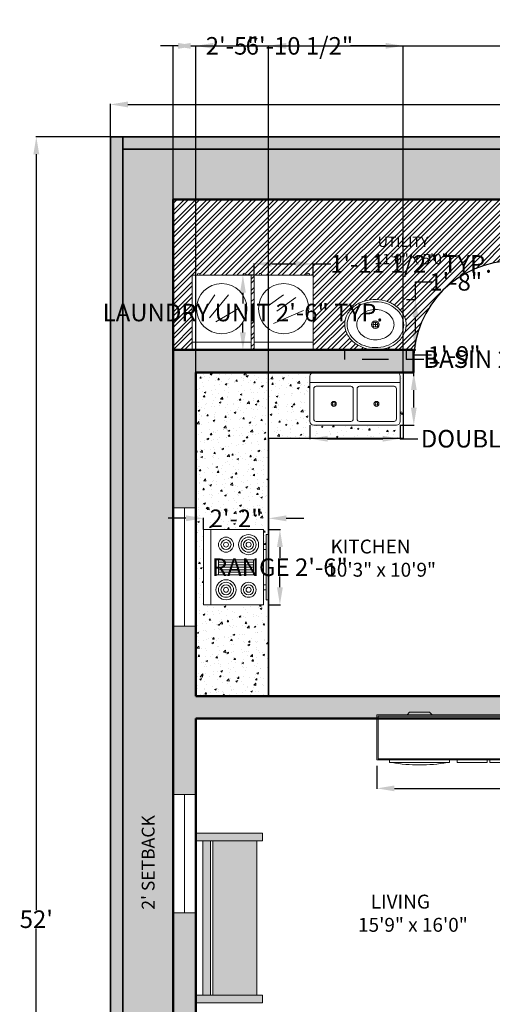
# Model space of a CAD drawing. Units: inches. Extents: x 319 to 870, y 210 to 995.
# Tile 4 of 6: x 336 to 524, y 603 to 995. Entities that reach past the tile are written whole.
import ezdxf

# ---------------------------------------------------------------- set-up
doc = ezdxf.new("R2010")
doc.units = ezdxf.units.IN
doc.header["$MEASUREMENT"] = 0
for name, color, linetype, lineweight in [('A-ANNO-DIMS', 2, 'Continuous', 18), ('A-ANNO-TEXT', 7, 'Continuous', 18), ('A-AREA-IDEN', 7, 'Continuous', 18), ('A-DOOR', 4, 'Continuous', 25), ('A-EQPM', 8, 'Continuous', 18), ('A-FLOR-CASE', 7, 'Continuous', 25), ('A-FLOR-CASE-PATT', 252, 'Continuous', 13), ('A-FLOR-FIXT', 9, 'Continuous', 18), ('A-FLOR-PATT', 252, 'Continuous', 13), ('A-FURN', 8, 'Continuous', 18), ('A-GLAZ', 4, 'Continuous', 18), ('A-WALL', 7, 'Continuous', 50), ('A-WALL-PATT', 8, 'Continuous', 13), ('C-PROP', 7, 'Continuous', 35), ('C-PROP-PATT', 8, 'Continuous', 13)]:
    doc.layers.add(name, color=color, linetype=linetype, lineweight=lineweight)
doc.layers.add('A-FURN-PATT', color=30, linetype='Continuous', lineweight=13, true_color=0xf7941d)
doc.layers.add('C-SITE-PATT', color=126, linetype='Continuous', lineweight=13, true_color=0x1e6f63)
doc.styles.get("Standard").update_dxf_attribs({"font": 'arial.ttf'})
doc.dimstyles.get("Standard").update_dxf_attribs({"dimtxt": 7, "dimasz": 7, "dimexe": 0.18, "dimexo": 0.0625, "dimgap": 0.09, "dimtad": 0, "dimtih": 1, "dimtoh": 1, "dimdec": 0, "dimzin": 0, "dimdsep": 46, "dimlunit": 3, "dimtxsty": 'Standard', "dimcen": 0.09, "dimadec": 0, "dimazin": 0, "dimtfac": 1, "dimtdec": 0, "dimtofl": 0, "dimtmove": 0, "dimatfit": 3, "dimfxl": 1, "dimtolj": 1, "dimtzin": 0, "dimarcsym": 0})

# ---------------------------------------------------------------- blocks, each defined once
blk = doc.blocks.new('Sink-double - 36 in top')
for p, q in [((-18, -4), (18, -4)), ((-0.75, -18.5), (-0.75, -6.5)), ((0.75, -6.5), (0.75, -18.5))]:
    blk.add_line(p, q)
for points in [[(-16.5, 0), (16.5, 0)], [(-18, -19.5), (-18, -1.5)], [(18, -1.5), (18, -19.5)], [(-16.5, -18.5), (-16.5, -6.5)], [(-15.5, -5.5), (-1.75, -5.5)], [(1.75, -5.5), (15.5, -5.5)], [(16.5, -6.5), (16.5, -18.5)], [(-1.75, -19.5), (-15.5, -19.5)], [(15.5, -19.5), (1.75, -19.5)], [(16.5, -21), (-16.5, -21)]]:
    blk.add_lwpolyline(points)
for centre, radius in [((-8.5, -12.5), 1), ((8.5, -12.5), 1), ((-8.5, -12.5), 0.5), ((8.5, -12.5), 0.5)]:
    blk.add_circle(centre, radius)
for centre, radius, start, end in [((-16.5, -1.5), 1.5, 90, 180), ((16.5, -1.5), 1.5, 0, 90), ((-15.5, -6.5), 1, 90, 180), ((-1.75, -6.5), 1, 0, 90), ((1.75, -6.5), 1, 90, 180), ((15.5, -6.5), 1, 0, 90), ((-16.5, -19.5), 1.5, 180, 270), ((-15.5, -18.5), 1, 180, 270), ((-1.75, -18.5), 1, 270, 0), ((1.75, -18.5), 1, 180, 270), ((15.5, -18.5), 1, 270, 0), ((16.5, -19.5), 1.5, 270, 0)]:
    blk.add_arc(centre, radius, start, end)
blk = doc.blocks.new('Range-Oven - 30 in top')
for p, q in [((0, -3), (30, -3)), ((12, -6), (18, -6)), ((13, -20), (13, -6)), ((14, -6), (14, -20)), ((15, -20), (15, -6)), ((16, -6), (16, -20)), ((17, -20), (17, -6)), ((18, -20), (12, -20)), ((6, -24), (6, -25)), ((8, -25), (8, -24)), ((22, -25), (22, -24)), ((24, -24), (24, -25))]:
    blk.add_line(p, q)
for points in [[(0, -24), (0, 0), (30, 0), (30, -24)], [(12, -21), (12, -5), (18, -5), (18, -21)], [(2, -26), (2, -25), (28, -25), (28, -26)]]:
    blk.add_lwpolyline(points, close=True)
for centre, radius in [((6, -9), 4), ((6, -9), 3), ((6, -9), 2), ((24, -9), 3), ((24, -9), 2), ((6, -9), 1), ((24, -9), 1), ((6, -18), 3), ((24, -18), 4), ((24, -18), 3), ((6, -18), 2), ((6, -18), 1), ((24, -18), 2), ((24, -18), 1)]:
    blk.add_circle(centre, radius)
blk = doc.blocks.new('Sink - Oval top')
for p, q in [((-1, 0), (1, 0)), ((0, 1), (0, -1))]:
    blk.add_line(p, q)
for points in [[(-12.23, 0.39, 0.117634), (-11.46, -3.36, 0.104469), (-8.88, -6.8, 0.090016), (-5.08, -9.07, 0.08192), (-0.32, -10.02, 0.08192), (4.49, -9.38, 0.090016), (8.42, -7.36, 0.104469), (11.22, -4.09, 0.117634), (12.23, -0.39, 0.117634), (11.46, 3.36, 0.104469), (8.88, 6.8, 0.090016), (5.08, 9.07, 0.08192), (0.32, 10.02, 0.08192), (-4.49, 9.38, 0.090016), (-8.42, 7.36, 0.104469), (-11.22, 4.09, 0.117634)], [(-11.29, 0.16, 0.118622), (-10.52, -3.25, 0.104678), (-8.07, -6.36, 0.089562), (-4.54, -8.37, 0.081185), (-0.13, -9.15, 0.081185), (4.3, -8.49, 0.089562), (7.89, -6.58, 0.104678), (10.42, -3.55, 0.118622), (11.29, -0.16, 0.118622), (10.52, 3.25, 0.104678), (8.07, 6.36, 0.089562), (4.54, 8.37, 0.081185), (0.13, 9.15, 0.081185), (-4.3, 8.49, 0.089562), (-7.89, 6.58, 0.104678), (-10.42, 3.55, 0.118622)], [(-7.42, 0.08, 0.118283), (-6.91, -2.17, 0.104607), (-5.29, -4.21, 0.089718), (-2.97, -5.53, 0.081436), (-0.07, -6.04, 0.081436), (2.84, -5.59, 0.089718), (5.2, -4.33, 0.104607), (6.86, -2.32, 0.118283), (7.42, -0.08, 0.118283), (6.91, 2.17, 0.104607), (5.29, 4.21, 0.089718), (2.97, 5.53, 0.081436), (0.07, 6.04, 0.081436), (-2.84, 5.59, 0.089718), (-5.2, 4.33, 0.104607), (-6.86, 2.32, 0.118283)]]:
    blk.add_lwpolyline(points, format="xyb", close=True)
for radius in [1.5, 1]:
    blk.add_circle((0, 0), radius)
blk = doc.blocks.new('*U12')
for p, q in [((0, 0), (0, -6)), ((-40, 0), (-40, -6))]:
    blk.add_line(p, q)
blk.add_lwpolyline([(0, 0), (0, 40), (-1.75, 40), (-1.75, 0)], close=True)
blk.add_arc((0, 0), 40, 90, 180)
blk = doc.blocks.new('Entertainment Center')
for p, q in [((-4, 0), (-5, -1)), ((4, 0), (-4, 0)), ((5, -1), (4, 0)), ((-17, -19), (-17, -1)), ((-17, -1), (43, -1)), ((-16.5, -18.5), (-16.5, -1.5)), ((-16.5, -1.5), (42.5, -1.5)), ((42.5, -1.5), (42.5, -18.5)), ((43, -1), (43, -19)), ((43, -19), (-17, -19)), ((42.5, -18.5), (-16.5, -18.5)), ((-12, -20), (-12, -19)), ((12, -19), (12, -20)), ((15, -20), (15, -19)), ((27, -19), (27, -20)), ((28, -20), (28, -19)), ((40, -19), (40, -20)), ((12, -20), (-12, -20)), ((27, -20), (15, -20)), ((40, -20), (28, -20))]:
    blk.add_line(p, q)
blk.add_arc((0, 40), 61, 259.6111, 280.3889)
blk = doc.blocks.new('*D22')
at = {"layer": 'A-ANNO-DIMS', "color": 0, "lineweight": -2, "transparency": 16777216}
for p, q in [((371.62, 948.67), (341.96, 948.67)), ((342.14, 941.67), (342.14, 640.33)), ((342.14, 331.67), (342.14, 633)), ((371.62, 324.67), (341.96, 324.67))]:
    blk.add_line(p, q, dxfattribs=at)
at = {"layer": 'A-ANNO-DIMS', "color": 0, "transparency": 16777216}
for points in [[(340.97, 941.67), (343.31, 941.67), (342.14, 948.67)], [(340.97, 331.67), (343.31, 331.67), (342.14, 324.67)]]:
    blk.add_solid(points, dxfattribs=at)
at = {"layer": 'Defpoints', "color": 0, "transparency": 16777216}
for p in [(371.68, 948.67), (342.14, 324.67), (371.68, 324.67)]:
    blk.add_point(p, dxfattribs=at)
at = {"layer": 'A-ANNO-DIMS', "color": 0, "transparency": 16777216, "insert": (342.14, 636.67), "char_height": 7, "attachment_point": 5}
blk.add_mtext("\\A1;52'", dxfattribs=at)
blk = doc.blocks.new('*D23')
at = {"layer": 'A-ANNO-DIMS', "color": 0, "lineweight": -2, "transparency": 16777216}
for p, q in [((371.68, 948.73), (371.68, 961.74)), ((378.68, 961.56), (575.66, 961.56)), ((784.68, 961.56), (587.71, 961.56)), ((791.68, 948.73), (791.68, 961.74))]:
    blk.add_line(p, q, dxfattribs=at)
at = {"layer": 'A-ANNO-DIMS', "color": 0, "transparency": 16777216}
for points in [[(378.68, 962.73), (378.68, 960.39), (371.68, 961.56)], [(784.68, 962.73), (784.68, 960.39), (791.68, 961.56)]]:
    blk.add_solid(points, dxfattribs=at)
at = {"layer": 'Defpoints', "color": 0, "transparency": 16777216}
for p in [(791.68, 961.56), (371.68, 948.67), (791.68, 948.67)]:
    blk.add_point(p, dxfattribs=at)
at = {"layer": 'A-ANNO-DIMS', "color": 0, "transparency": 16777216, "insert": (581.68, 961.56), "char_height": 7, "attachment_point": 5}
blk.add_mtext("\\A1;35'", dxfattribs=at)
blk = doc.blocks.new('EQPM-LAUNDRY-CABINET-DRUM')
for p, q in [((0, 0), (0, 29.82)), ((0, 29.82), (23.57, 29.82)), ((23.57, 29.82), (23.57, 0)), ((23.57, 3.06), (0, 3.06))]:
    blk.add_line(p, q)
blk.add_circle((11.78, 16.44), 10.02)
blk = doc.blocks.new('*D29')
at = {"layer": 'A-ANNO-DIMS', "color": 0, "lineweight": -2, "transparency": 16777216}
for p, q in [((477.94, 697.77), (477.94, 688.66)), ((537.94, 697.77), (537.94, 688.66)), ((484.94, 688.84), (530.94, 688.84)), ((537.94, 688.84), (544.94, 688.84))]:
    blk.add_line(p, q, dxfattribs=at)
at = {"layer": 'A-ANNO-DIMS', "color": 0, "transparency": 16777216}
for points in [[(484.94, 690), (484.94, 687.67), (477.94, 688.84)], [(530.94, 690), (530.94, 687.67), (537.94, 688.84)]]:
    blk.add_solid(points, dxfattribs=at)
at = {"layer": 'Defpoints', "color": 0, "transparency": 16777216}
for p in [(477.94, 697.84), (537.94, 697.84), (537.94, 688.84)]:
    blk.add_point(p, dxfattribs=at)
at = {"layer": 'A-ANNO-DIMS', "color": 0, "transparency": 16777216, "insert": (595.82, 688.84), "char_height": 7, "attachment_point": 5}
blk.add_mtext('\\A1;MEDIA UNIT 5\'-0" TYP.', dxfattribs=at)
blk = doc.blocks.new('*D41')
at = {"layer": 'A-ANNO-DIMS', "color": 0, "lineweight": -2, "transparency": 16777216}
for p, q in [((428.91, 893.49), (424.32, 893.49)), ((424.5, 886.49), (424.5, 882.24)), ((424.5, 870.67), (424.5, 874.92)), ((428.91, 863.67), (424.32, 863.67))]:
    blk.add_line(p, q, dxfattribs=at)
at = {"layer": 'A-ANNO-DIMS', "color": 0, "transparency": 16777216}
for points in [[(423.34, 886.49), (425.67, 886.49), (424.5, 893.49)], [(423.34, 870.67), (425.67, 870.67), (424.5, 863.67)]]:
    blk.add_solid(points, dxfattribs=at)
at = {"layer": 'Defpoints', "color": 0, "transparency": 16777216}
for p in [(424.5, 893.49), (428.98, 893.49), (428.98, 863.67)]:
    blk.add_point(p, dxfattribs=at)
at = {"layer": 'A-ANNO-DIMS', "color": 0, "transparency": 16777216, "insert": (424.5, 878.58), "char_height": 7, "attachment_point": 5}
blk.add_mtext('\\A1;LAUNDRY UNIT 2\'-6" TYP.', dxfattribs=at)
blk = doc.blocks.new('*D42')
at = {"layer": 'A-ANNO-DIMS', "color": 0, "lineweight": -2, "transparency": 16777216}
for p, q in [((428.98, 893.55), (428.98, 898.15)), ((435.98, 897.97), (445.54, 897.97)), ((452.54, 893.55), (452.54, 898.15)), ((452.54, 897.97), (459.54, 897.97))]:
    blk.add_line(p, q, dxfattribs=at)
at = {"layer": 'A-ANNO-DIMS', "color": 0, "transparency": 16777216}
for points in [[(435.98, 899.13), (435.98, 896.8), (428.98, 897.97)], [(445.54, 899.13), (445.54, 896.8), (452.54, 897.97)]]:
    blk.add_solid(points, dxfattribs=at)
at = {"layer": 'Defpoints', "color": 0, "transparency": 16777216}
for p in [(452.54, 897.97), (428.98, 893.49), (452.54, 893.49)]:
    blk.add_point(p, dxfattribs=at)
at = {"layer": 'A-ANNO-DIMS', "color": 0, "transparency": 16777216, "insert": (491.51, 897.97), "char_height": 7, "attachment_point": 5}
blk.add_mtext('\\A1;1\'-11 1/2" TYP.', dxfattribs=at)
blk = doc.blocks.new('*D43')
at = {"layer": 'A-ANNO-DIMS', "color": 0, "lineweight": -2, "transparency": 16777216}
for p, q in [((451.25, 833.61), (451.25, 828.09)), ((487.25, 833.61), (487.25, 828.09)), ((458.25, 828.27), (480.25, 828.27)), ((487.25, 828.27), (494.25, 828.27))]:
    blk.add_line(p, q, dxfattribs=at)
at = {"layer": 'A-ANNO-DIMS', "color": 0, "transparency": 16777216}
for points in [[(458.25, 829.44), (458.25, 827.1), (451.25, 828.27)], [(480.25, 829.44), (480.25, 827.1), (487.25, 828.27)]]:
    blk.add_solid(points, dxfattribs=at)
at = {"layer": 'Defpoints', "color": 0, "transparency": 16777216}
for p in [(451.25, 833.67), (487.25, 833.67), (487.25, 828.27)]:
    blk.add_point(p, dxfattribs=at)
at = {"layer": 'A-ANNO-DIMS', "color": 0, "transparency": 16777216, "insert": (537.71, 828.27), "char_height": 7, "attachment_point": 5}
blk.add_mtext('\\A1;DOUBLE SINK 3\'-0"', dxfattribs=at)
blk = doc.blocks.new('*D44')
at = {"layer": 'A-ANNO-DIMS', "color": 0, "lineweight": -2, "transparency": 16777216}
for p, q in [((492.65, 854.67), (492.65, 861.67)), ((492.65, 861.67), (499.65, 861.67)), ((487.31, 854.67), (492.83, 854.67)), ((492.65, 840.67), (492.65, 847.67)), ((487.31, 833.67), (492.83, 833.67))]:
    blk.add_line(p, q, dxfattribs=at)
at = {"layer": 'A-ANNO-DIMS', "color": 0, "transparency": 16777216}
for points in [[(491.49, 847.67), (493.82, 847.67), (492.65, 854.67)], [(491.49, 840.67), (493.82, 840.67), (492.65, 833.67)]]:
    blk.add_solid(points, dxfattribs=at)
at = {"layer": 'Defpoints', "color": 0, "transparency": 16777216}
for p in [(487.25, 854.67), (492.65, 854.67), (487.25, 833.67)]:
    blk.add_point(p, dxfattribs=at)
at = {"layer": 'A-ANNO-DIMS', "color": 0, "transparency": 16777216, "insert": (508.72, 861.67), "char_height": 7, "attachment_point": 5}
blk.add_mtext('\\A1;1\'-9"', dxfattribs=at)
blk = doc.blocks.new('*D45')
at = {"layer": 'A-ANNO-DIMS', "color": 0, "lineweight": -2, "transparency": 16777216}
for p, q in [((434.83, 792.03), (439.45, 792.03)), ((439.27, 785.03), (439.27, 780.74)), ((439.27, 769.03), (439.27, 773.32)), ((434.83, 762.03), (439.45, 762.03))]:
    blk.add_line(p, q, dxfattribs=at)
at = {"layer": 'A-ANNO-DIMS', "color": 0, "transparency": 16777216}
for points in [[(438.1, 785.03), (440.44, 785.03), (439.27, 792.03)], [(438.1, 769.03), (440.44, 769.03), (439.27, 762.03)]]:
    blk.add_solid(points, dxfattribs=at)
at = {"layer": 'Defpoints', "color": 0, "transparency": 16777216}
for p in [(434.77, 792.03), (439.27, 792.03), (434.77, 762.03)]:
    blk.add_point(p, dxfattribs=at)
at = {"layer": 'A-ANNO-DIMS', "color": 0, "transparency": 16777216, "insert": (439.27, 777.03), "char_height": 7, "attachment_point": 5}
blk.add_mtext('\\A1;RANGE 2\'-6"', dxfattribs=at)
blk = doc.blocks.new('*D46')
at = {"layer": 'A-ANNO-DIMS', "color": 0, "lineweight": -2, "transparency": 16777216}
for p, q in [((401.77, 796.53), (394.77, 796.53)), ((408.77, 792.09), (408.77, 796.71)), ((434.77, 792.09), (434.77, 796.71)), ((441.77, 796.53), (448.77, 796.53))]:
    blk.add_line(p, q, dxfattribs=at)
at = {"layer": 'A-ANNO-DIMS', "color": 0, "transparency": 16777216}
for points in [[(401.77, 797.7), (401.77, 795.36), (408.77, 796.53)], [(441.77, 797.7), (441.77, 795.36), (434.77, 796.53)]]:
    blk.add_solid(points, dxfattribs=at)
at = {"layer": 'Defpoints', "color": 0, "transparency": 16777216}
for p in [(408.77, 796.53), (408.77, 792.03), (434.77, 792.03)]:
    blk.add_point(p, dxfattribs=at)
at = {"layer": 'A-ANNO-DIMS', "color": 0, "transparency": 16777216, "insert": (421.77, 796.53), "char_height": 7, "attachment_point": 5}
blk.add_mtext('\\A1;2\'-2"', dxfattribs=at)
blk = doc.blocks.new('*D47')
at = {"layer": 'A-ANNO-DIMS', "color": 0, "lineweight": -2, "transparency": 16777216}
for p, q in [((465.06, 863.63), (465.06, 859.83)), ((472.06, 860.01), (482.61, 860.01)), ((489.61, 863.63), (489.61, 859.83)), ((489.61, 860.01), (496.61, 860.01))]:
    blk.add_line(p, q, dxfattribs=at)
at = {"layer": 'A-ANNO-DIMS', "color": 0, "transparency": 16777216}
for points in [[(472.06, 861.17), (472.06, 858.84), (465.06, 860.01)], [(482.61, 861.17), (482.61, 858.84), (489.61, 860.01)]]:
    blk.add_solid(points, dxfattribs=at)
at = {"layer": 'Defpoints', "color": 0, "transparency": 16777216}
for p in [(465.06, 863.69), (489.61, 863.69), (489.61, 860.01)]:
    blk.add_point(p, dxfattribs=at)
at = {"layer": 'A-ANNO-DIMS', "color": 0, "transparency": 16777216, "insert": (530.04, 860.01), "char_height": 7, "attachment_point": 5}
blk.add_mtext('\\A1;BASIN 2\'-0 1/2"', dxfattribs=at)
blk = doc.blocks.new('*D48')
at = {"layer": 'A-ANNO-DIMS', "color": 0, "lineweight": -2, "transparency": 16777216}
for p, q in [((493.3, 883.83), (493.3, 890.83)), ((493.3, 890.83), (500.3, 890.83)), ((489.68, 883.83), (493.48, 883.83)), ((493.3, 870.69), (493.3, 876.83)), ((489.68, 863.69), (493.48, 863.69))]:
    blk.add_line(p, q, dxfattribs=at)
at = {"layer": 'A-ANNO-DIMS', "color": 0, "transparency": 16777216}
for points in [[(492.13, 876.83), (494.46, 876.83), (493.3, 883.83)], [(492.13, 870.69), (494.46, 870.69), (493.3, 863.69)]]:
    blk.add_solid(points, dxfattribs=at)
at = {"layer": 'Defpoints', "color": 0, "transparency": 16777216}
for p in [(489.61, 883.83), (493.3, 883.83), (489.61, 863.69)]:
    blk.add_point(p, dxfattribs=at)
at = {"layer": 'A-ANNO-DIMS', "color": 0, "transparency": 16777216, "insert": (509.36, 890.83), "char_height": 7, "attachment_point": 5}
blk.add_mtext('\\A1;1\'-8"', dxfattribs=at)
blk = doc.blocks.new('*D49')
at = {"layer": 'A-ANNO-DIMS', "color": 0, "lineweight": -2, "transparency": 16777216}
for p, q in [((396.68, 923.73), (396.68, 985.1)), ((403.68, 984.92), (566.85, 984.92)), ((759.68, 984.92), (596.52, 984.92)), ((766.68, 923.73), (766.68, 985.1))]:
    blk.add_line(p, q, dxfattribs=at)
at = {"layer": 'A-ANNO-DIMS', "color": 0, "transparency": 16777216}
for points in [[(403.68, 986.09), (403.68, 983.75), (396.68, 984.92)], [(759.68, 986.09), (759.68, 983.75), (766.68, 984.92)]]:
    blk.add_solid(points, dxfattribs=at)
at = {"layer": 'Defpoints', "color": 0, "transparency": 16777216}
for p in [(766.68, 984.92), (396.68, 923.67), (766.68, 923.67)]:
    blk.add_point(p, dxfattribs=at)
at = {"layer": 'A-ANNO-DIMS', "color": 0, "transparency": 16777216, "insert": (581.68, 984.92), "char_height": 7, "attachment_point": 5}
blk.add_mtext('\\A1;30\'-10"', dxfattribs=at)
blk = doc.blocks.new('*D57')
at = {"layer": 'A-ANNO-DIMS', "color": 0, "lineweight": -2, "transparency": 16777216}
for p, q in [((405.68, 854.73), (405.68, 985.1)), ((412.68, 984.92), (426.76, 984.92)), ((481.42, 984.92), (467.34, 984.92)), ((488.42, 854.73), (488.42, 985.1))]:
    blk.add_line(p, q, dxfattribs=at)
at = {"layer": 'A-ANNO-DIMS', "color": 0, "transparency": 16777216}
for points in [[(412.68, 986.09), (412.68, 983.75), (405.68, 984.92)], [(481.42, 986.09), (481.42, 983.75), (488.42, 984.92)]]:
    blk.add_solid(points, dxfattribs=at)
at = {"layer": 'Defpoints', "color": 0, "transparency": 16777216}
for p in [(488.42, 984.92), (405.68, 854.67), (488.42, 854.67)]:
    blk.add_point(p, dxfattribs=at)
at = {"layer": 'A-ANNO-DIMS', "color": 0, "transparency": 16777216, "insert": (447.05, 984.92), "char_height": 7, "attachment_point": 5}
blk.add_mtext('\\A1;6\'-10 1/2"', dxfattribs=at)
blk = doc.blocks.new('*D58')
at = {"layer": 'A-ANNO-DIMS', "color": 0, "lineweight": -2, "transparency": 16777216}
for p, q in [((398.68, 984.92), (391.68, 984.92)), ((405.68, 725.73), (405.68, 985.1)), ((434.77, 725.73), (434.77, 985.1)), ((441.77, 984.92), (448.77, 984.92))]:
    blk.add_line(p, q, dxfattribs=at)
at = {"layer": 'A-ANNO-DIMS', "color": 0, "transparency": 16777216}
for points in [[(398.68, 986.09), (398.68, 983.75), (405.68, 984.92)], [(441.77, 986.09), (441.77, 983.75), (434.77, 984.92)]]:
    blk.add_solid(points, dxfattribs=at)
at = {"layer": 'Defpoints', "color": 0, "transparency": 16777216}
for p in [(434.77, 984.92), (405.68, 725.67), (434.77, 725.67)]:
    blk.add_point(p, dxfattribs=at)
at = {"layer": 'A-ANNO-DIMS', "color": 0, "transparency": 16777216, "insert": (420.23, 984.92), "char_height": 7, "attachment_point": 5}
blk.add_mtext('\\A1;2\'-5"', dxfattribs=at)

msp = doc.modelspace()

# ---------------------------------------------------------------- hatches: boundary and pattern name
at = {"layer": 'A-FLOR-CASE-PATT'}
h = msp.add_hatch(dxfattribs=at)
h.set_pattern_fill('AR-CONC', color=256)
h.set_pattern_definition([(50, (0, 0), (7.172602, -0.62752), [0.75, -8.25]), (355, (0, 0), (-1.387513, 7.52192), [0.6, -6.6]), (100.45144, (0.598, -0.052), (5.78509, 6.8944), [0.6374, -7.01142]), (46.1842, (0, 2), (10.67241, -1.65519), [1.125, -12.375]), (96.6356, (0.889, 1.862), (9.34662, 9.74119), [0.9561, -10.51714]), (351.1842, (0, 2), (9.34662, 9.74119), [0.9, -9.9]), (21, (1, 1.5), (5.96907, -4.02619), [0.75, -8.25]), (326, (1, 1.5), (2.433153, 7.2515), [0.6, -6.6]), (71.45144, (1.4974, 1.1645), (8.402224, 3.22531), [0.6374, -7.01142]), (37.5, (0, 0), (0.1215986, 3.3289385), [0, -6.52, 0, -6.7, 0, -6.625]), (7.5, (0, 0), (2.630695, 3.944117), [0, -3.82, 0, -6.37, 0, -2.525]), (327.5, (-2.23, 0), (5.338224, -0.225549), [0, -2.5, 0, -7.8, 0, -10.35]), (317.5, (-3.23, 0), (5.831862, 1.00105), [0, -3.25, 0, -5.18, 0, -7.35])])
h.paths.add_polyline_path([(405.68, 725.67), (434.77, 725.67), (434.77, 764.03), (433.77, 764.03), (433.77, 768.03), (432.77, 768.03), (432.77, 762.03), (408.77, 762.03), (408.77, 792.03), (432.77, 792.03), (432.77, 786.03), (433.77, 786.03), (433.77, 790.03), (434.77, 790.03), (434.77, 828.39), (488.42, 828.39), (488.42, 854.67), (485.75, 854.67, -0.414214), (487.25, 853.17), (487.25, 835.17, -0.414214), (485.75, 833.67), (452.75, 833.67, -0.414214), (451.25, 835.17), (451.25, 853.17, -0.414214), (452.75, 854.67), (405.68, 854.67)])
at = {"layer": 'A-FLOR-PATT'}
h = msp.add_hatch(dxfattribs=at)
h.set_pattern_fill('STEEL', color=256)
h.set_pattern_definition([(45, (0, 0), (-2.245064, 2.245064), []), (45, (0, 1.5875), (-2.245064, 2.245064), [])])
h.paths.add_polyline_path([(472.85, 883.14, -0.08192), (477.66, 883.77, -0.08192), (482.42, 882.83, -0.090016), (486.22, 880.56, -0.104469), (488.8, 877.12, -0.117634), (489.57, 873.36, -0.117634), (488.56, 869.67, -0.104469), (485.76, 866.4, -0.090016), (481.83, 864.38, -0.073818), (477.49, 863.73), (492.56, 863.67), (492.82, 863.67, -0.354003), (528.68, 898.98), (528.68, 923.67), (396.68, 923.67), (396.68, 863.67), (404.28, 863.67), (404.28, 893.49), (406.44, 893.49, -1.658066), (407.33, 893.49), (424.73, 893.49, -1.757253), (425.6, 893.49), (427.85, 893.49), (427.85, 863.67), (428.98, 863.67), (428.98, 893.49), (431.02, 893.49, -1.575486), (431.93, 893.49), (450.07, 893.49, -1.717768), (450.95, 893.49), (452.54, 893.49), (452.54, 863.67), (477.49, 863.73, -0.008053), (477.01, 863.74, -0.08192), (472.25, 864.69, -0.090016), (468.46, 866.95, -0.104469), (465.87, 870.4, -0.117634), (465.1, 874.15, -0.117634), (466.11, 877.85, -0.104469), (468.92, 881.12, -0.090016)])
h.paths.add_polyline_path([(475.31, 895.58), (505.85, 895.58), (505.85, 911.01), (475.31, 911.01)], flags=24)
at = {"layer": 'A-FURN-PATT'}
h = msp.add_hatch(color=256, dxfattribs=at)
h.dxf.hatch_style = 1
h.paths.add_polyline_path([(432.33, 667.94), (432.33, 670.94), (405.68, 670.94), (405.68, 667.94)])
h = msp.add_hatch(color=256, dxfattribs=at)
h.dxf.hatch_style = 1
h.paths.add_polyline_path([(411.58, 667.94), (408.53, 667.94), (408.53, 606.35), (411.58, 606.35)])
h = msp.add_hatch(color=256, dxfattribs=at)
h.dxf.hatch_style = 1
h.paths.add_polyline_path([(412.58, 606.35), (430.1, 606.35), (430.1, 667.94), (412.58, 667.94)])
h = msp.add_hatch(color=256, dxfattribs=at)
h.dxf.hatch_style = 1
h.paths.add_polyline_path([(432.33, 603.35), (432.33, 606.35), (405.68, 606.35), (405.68, 603.35)])
at = {"layer": 'A-WALL-PATT'}
h = msp.add_hatch(color=256, dxfattribs=at)
h.dxf.hatch_style = 1
h.paths.add_polyline_path([(396.68, 863.67), (396.68, 800.7), (405.68, 800.7), (405.68, 854.67), (492.56, 854.67), (492.56, 863.67)])
h = msp.add_hatch(color=256, dxfattribs=at)
h.dxf.hatch_style = 1
h.paths.add_polyline_path([(405.68, 725.67), (405.68, 753.49), (396.68, 753.49), (396.68, 686.41), (405.68, 686.41), (405.68, 716.67), (537.68, 716.67), (559.06, 716.67), (559.06, 725.67), (528.68, 725.67)])
h = msp.add_hatch(color=256, dxfattribs=at)
h.dxf.hatch_style = 1
h.paths.add_polyline_path([(396.68, 590.1), (405.68, 590.1), (405.68, 639.21), (396.68, 639.21)])
at = {"layer": 'C-PROP-PATT'}
h = msp.add_hatch(color=256, dxfattribs=at)
h.dxf.hatch_style = 1
h.paths.add_polyline_path([(371.68, 324.67), (391.35, 324.67), (391.35, 329.67), (376.68, 329.67), (376.68, 948.67), (371.68, 948.67)])
h = msp.add_hatch(color=256, dxfattribs=at)
h.dxf.hatch_style = 1
h.paths.add_polyline_path([(757.68, 329.67), (597.68, 329.67), (597.68, 324.67), (791.68, 324.67), (791.68, 948.67), (376.68, 948.67), (376.68, 943.67), (786.68, 943.67), (786.68, 329.67), (766.68, 329.67), (766.68, 354.04), (757.68, 354.04)])
at = {"layer": 'C-SITE-PATT'}
h = msp.add_hatch(color=256, dxfattribs=at)
h.dxf.hatch_style = 1
h.paths.add_polyline_path([(376.68, 515.67), (396.68, 515.67), (396.68, 923.67), (528.68, 923.67), (606.68, 923.67), (766.68, 923.67), (766.68, 329.67), (786.68, 329.67), (786.68, 943.67), (376.68, 943.67)])
h.paths.add_polyline_path([(392.17, 638.98), (392.17, 682.3), (381.61, 682.3), (381.61, 638.98)], flags=24)
h.paths.add_polyline_path([(772.77, 716.95), (772.77, 673.64), (783.33, 673.64), (783.33, 716.95)], flags=24)
h.paths.add_polyline_path([(542.27, 929.56), (581.61, 929.56), (581.61, 939.15), (542.27, 939.15)], flags=24)

# ---------------------------------------------------------------- linework, layer by layer
at = {"layer": 'A-EQPM'}
for p, q in [((413.28, 885.59), (409.32, 879.69)), ((418.77, 885.67), (411.17, 876.48)), ((440.7, 885.59), (434.63, 881.2)), ((445.6, 884.58), (438, 879.1)), ((423.07, 880.36), (413.7, 874.88)), ((448.72, 879.43), (436.65, 874.21))]:
    msp.add_line(p, q, dxfattribs=at)
for centre in [(406.88, 893.73), (425.16, 893.75), (431.48, 893.71), (450.51, 893.74)]:
    msp.add_arc(centre, 0.501, 332.1894, 207.8106, dxfattribs=at)
at = {"layer": 'A-FLOR-CASE'}
for p, q in [((488.42, 854.67), (488.42, 828.39)), ((488.42, 828.39), (434.77, 828.39)), ((434.77, 828.39), (434.77, 725.67))]:
    msp.add_line(p, q, dxfattribs=at)
at = {"layer": 'A-FURN'}
for p, q in [((432.33, 670.94), (405.68, 670.94)), ((432.33, 667.94), (405.68, 667.94)), ((408.53, 667.94), (408.53, 606.35)), ((411.58, 667.94), (411.58, 606.35)), ((412.58, 667.94), (412.58, 606.35)), ((430.1, 667.94), (430.1, 606.35)), ((432.33, 670.94), (432.33, 667.94)), ((432.33, 606.35), (405.68, 606.35)), ((432.33, 603.35), (432.33, 606.35)), ((405.68, 603.35), (432.33, 603.35))]:
    msp.add_line(p, q, dxfattribs=at)
at = {"layer": 'A-GLAZ'}
for p, q in [((396.68, 800.7), (405.68, 800.7)), ((401.18, 800.7), (401.18, 753.49)), ((405.68, 753.49), (396.68, 753.49)), ((405.68, 686.41), (396.68, 686.41)), ((401.18, 639.21), (401.18, 686.41)), ((405.68, 639.21), (396.68, 639.21))]:
    msp.add_line(p, q, dxfattribs=at)
at = {"layer": 'A-WALL'}
for p, q in [((396.68, 923.67), (396.68, 515.67)), ((528.68, 923.67), (396.68, 923.67)), ((492.56, 863.67), (396.68, 863.67)), ((492.56, 863.67), (492.56, 854.67)), ((405.68, 854.67), (405.68, 725.67)), ((492.56, 854.67), (405.68, 854.67)), ((528.68, 725.67), (405.68, 725.67)), ((537.68, 716.67), (405.68, 716.67)), ((405.68, 716.67), (405.68, 524.67))]:
    msp.add_line(p, q, dxfattribs=at)
at = {"layer": 'C-PROP'}
for p, q in [((791.68, 948.67), (371.68, 948.67)), ((371.68, 948.67), (371.68, 324.67)), ((376.68, 948.67), (376.68, 329.67)), ((786.68, 943.67), (376.68, 943.67))]:
    msp.add_line(p, q, dxfattribs=at)

# ---------------------------------------------------------------- block references
at = {"layer": 'A-DOOR'}
msp.add_blockref('*U12', (532.56, 859.17), dxfattribs=at)
at = {"layer": 'A-EQPM'}
for p in [(404.28, 863.67), (428.98, 863.67)]:
    msp.add_blockref('EQPM-LAUNDRY-CABINET-DRUM', p, dxfattribs=at)
at = {"layer": 'A-EQPM', "rotation": 90}
msp.add_blockref('Range-Oven - 30 in top', (408.77, 762.03), dxfattribs=at)
at = {"layer": 'A-FLOR-FIXT'}
for name, p in [('Sink - Oval top', (477.34, 873.76)), ('Sink-double - 36 in top', (469.25, 854.67))]:
    msp.add_blockref(name, p, dxfattribs=at)
at = {"layer": 'A-FURN'}
msp.add_blockref('Entertainment Center', (494.94, 719.17), dxfattribs=at)

# ---------------------------------------------------------------- texts
at = {"layer": 'A-ANNO-TEXT', "insert": (384.16, 640.47), "char_height": 5.1244, "attachment_point": 1, "rotation": 90}
msp.add_mtext_dynamic_manual_height_columns("2' SETBACK ", width=66.3636, gutter_width=25.62, heights=[0], dxfattribs=at)
at = {"layer": 'A-AREA-IDEN', "attachment_point": 1}
for s, width, gutter_width, insert, char_height in [(' UTILITY\\P11\'0" x 5\'0"', 53.5592, 20.68, (476.98, 908.88), 4.1357), (' KITCHEN\\P10\'3" x 10\'9"', 71.8522, 27.74, (457.74, 788.05), 5.5482), ('   LIVING\\P15\'9" x 16\'0"', 71.8522, 27.74, (470.41, 646.46), 5.5482)]:
    msp.add_mtext_dynamic_manual_height_columns(s, width=width, gutter_width=gutter_width, heights=[0], dxfattribs=dict(at, insert=insert, char_height=char_height))

# ---------------------------------------------------------------- dimensions: what is measured, and where the dimension line sits
at = {"layer": 'A-ANNO-DIMS'}
for base, p1, p2, override, picture, middle in [((488.42, 984.92), (405.68, 854.67), (488.42, 854.67), {"dimdec": 1, "dimlfac": 1, "dimrnd": 0, "dimzin": 1, "dimdsep": 46, "dimlunit": 4, "dimfrac": 2}, '*D57', (447.05, 984.92)), ((434.77, 984.92), (405.68, 725.67), (434.77, 725.67), {"dimdec": 1, "dimlfac": 1, "dimrnd": 0, "dimzin": 1, "dimdsep": 46, "dimlunit": 4, "dimfrac": 2}, '*D58', (420.23, 984.92)), ((766.68, 984.92), (396.68, 923.67), (766.68, 923.67), {"dimdec": 1, "dimlfac": 1, "dimrnd": 0, "dimzin": 1, "dimdsep": 46, "dimlunit": 4, "dimfrac": 2}, '*D49', (581.68, 984.92)), ((791.68, 961.56), (371.68, 948.67), (791.68, 948.67), {"dimclrd": 0, "dimclre": 0, "dimclrt": 0}, '*D23', (581.68, 961.56))]:
    dim = msp.add_linear_dim(base=base, p1=p1, p2=p2, dimstyle='Standard', override=override, dxfattribs=at)
    dim.commit()
    dim.dimension.update_dxf_attribs({"geometry": picture, "text_midpoint": middle})
for base, p1, p2, angle, override, picture, middle in [((342.14, 324.67), (371.68, 948.67), (371.68, 324.67), 90, {"dimclrd": 0, "dimclre": 0, "dimclrt": 0}, '*D22', (342.14, 636.67)), ((493.3, 883.83), (489.61, 863.69), (489.61, 883.83), 90, {"dimdec": 1, "dimlfac": 1, "dimrnd": 0, "dimzin": 1, "dimdsep": 46, "dimlunit": 4, "dimfrac": 2}, '*D48', (509.36, 890.83)), ((492.65, 854.67), (487.25, 833.67), (487.25, 854.67), 90, {"dimdec": 1, "dimlfac": 1, "dimrnd": 0, "dimzin": 1, "dimdsep": 46, "dimlunit": 4, "dimfrac": 2}, '*D44', (508.72, 861.67)), ((408.77, 796.53), (434.77, 792.03), (408.77, 792.03), 180, {"dimdec": 1, "dimlfac": 1, "dimrnd": 0, "dimzin": 1, "dimdsep": 46, "dimlunit": 4, "dimfrac": 2}, '*D46', (421.77, 796.53))]:
    dim = msp.add_linear_dim(base=base, p1=p1, p2=p2, angle=angle, dimstyle='Standard', override=override, dxfattribs=at)
    dim.commit()
    dim.dimension.update_dxf_attribs({"geometry": picture, "text_midpoint": middle})
for base, p1, p2, text, picture, middle in [((452.54, 897.97), (428.98, 893.49), (452.54, 893.49), '<> TYP.', '*D42', (491.51, 897.97)), ((489.6129, 860.0071), (465.0621, 863.6897), (489.6129, 863.6897), 'BASIN <>', '*D47', (530.0389, 860.0071)), ((487.25, 828.27), (451.25, 833.67), (487.25, 833.67), 'DOUBLE SINK <>', '*D43', (537.71, 828.27)), ((537.94, 688.84), (477.94, 697.84), (537.94, 697.84), 'MEDIA UNIT <> TYP.', '*D29', (595.82, 688.84))]:
    dim = msp.add_linear_dim(base=base, p1=p1, p2=p2, text=text, dimstyle='Standard', override={"dimdec": 1, "dimlfac": 1, "dimrnd": 0, "dimzin": 1, "dimdsep": 46, "dimlunit": 4, "dimfrac": 2}, dxfattribs=at)
    dim.commit()
    dim.dimension.update_dxf_attribs({"geometry": picture, "text_midpoint": middle})
for base, p1, p2, text, picture, middle in [((424.5, 893.49), (428.98, 863.67), (428.98, 893.49), 'LAUNDRY UNIT <> TYP.', '*D41', (424.5, 878.58)), ((439.27, 792.03), (434.77, 762.03), (434.77, 792.03), 'RANGE <>', '*D45', (439.27, 777.03))]:
    dim = msp.add_linear_dim(base=base, p1=p1, p2=p2, angle=90, text=text, dimstyle='Standard', override={"dimdec": 1, "dimlfac": 1, "dimrnd": 0, "dimzin": 1, "dimdsep": 46, "dimlunit": 4, "dimfrac": 2}, dxfattribs=at)
    dim.commit()
    dim.dimension.update_dxf_attribs({"geometry": picture, "text_midpoint": middle})

doc.saveas('drawing.dxf')
